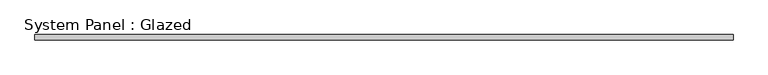
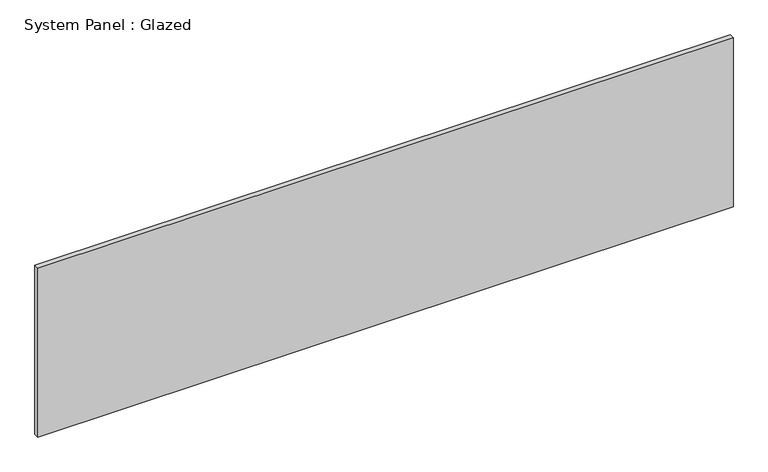
"""IFC4 building model written with IfcOpenShell, lengths in millimetres: plate geometry, System Panel : Glazed."""

from ifc_helpers import new_model, si_unit, origin, origin_with_axes, place, context, project, spatial, polyline, outline, extrude, source, transform, mapped, element, save


def system_panel_glazed_ef8a7044(model_context):
    return source(origin(), model_context, "Body", "SweptSolid", [
        extrude(outline(polyline([(1670.3270964, 19.05), (-1670.3270964, 19.05), (-1670.3270964, 44.45), (1670.3270964, 44.45), (1670.3270964, 19.05)])), origin_with_axes(), (0.0, 0.0, 1.0), 858.3570326),
    ])


if __name__ == "__main__":
    model = new_model("IFC4")
    model_context = context("Model", 3, world=origin())
    ifc_project = project(units=[si_unit("LENGTHUNIT", "METRE", prefix="MILLI")], contexts=[model_context])
    site = spatial("IfcSite", under=ifc_project)
    building = spatial("IfcBuilding", under=site)
    placement = place(None, origin())
    system_panel_glazed_shape = system_panel_glazed_ef8a7044(model_context)
    element("IfcPlate", 1, ObjectType="System Panel : Glazed", at=placement, inside=building, context=model_context, shape_type="MappedRepresentation", body=[
        mapped(system_panel_glazed_shape, transform((0.0, 0.0, 0.0), x_axis=(1.0, 0.0, 0.0), y_axis=(0.0, 1.0, 0.0), z_axis=(0.0, 0.0, 1.0))),
    ])
    save(model, "model.ifc")

# Revit data of these elements
# Type "System Panel : Glazed"
#   Construction Type Id = "GSP4R"
#   Analytic Construction = "1/8 in Pilkington single glazing"
#   Visual Light Transmittance = 0.9
#   Solar Heat Gain Coefficient = 0.86
#   Heat Transfer Coefficient (U) = 1.18115 BTU/(h·ft²·°F)
#   Define Thermal Properties by = 1
# Element 1 (IfcPlate, "System Panel : Glazed")
#   Materials on its faces: "Glass"
# Materials
#   "Glass": class "Glass", colour RGB 0 128 192, transparency 0.75, Description = "Soda Lime Glass", Cost = 0
